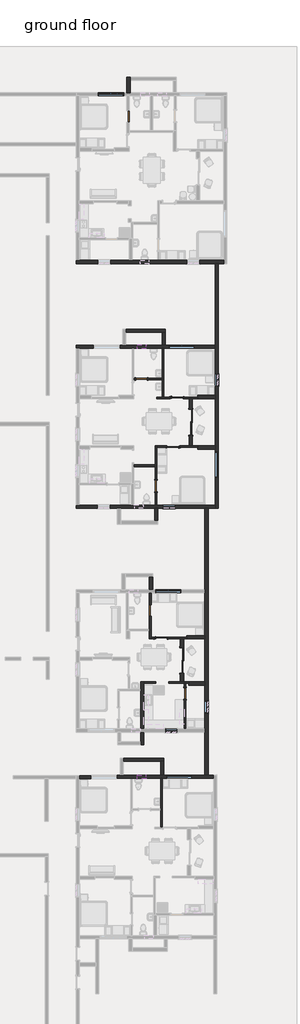
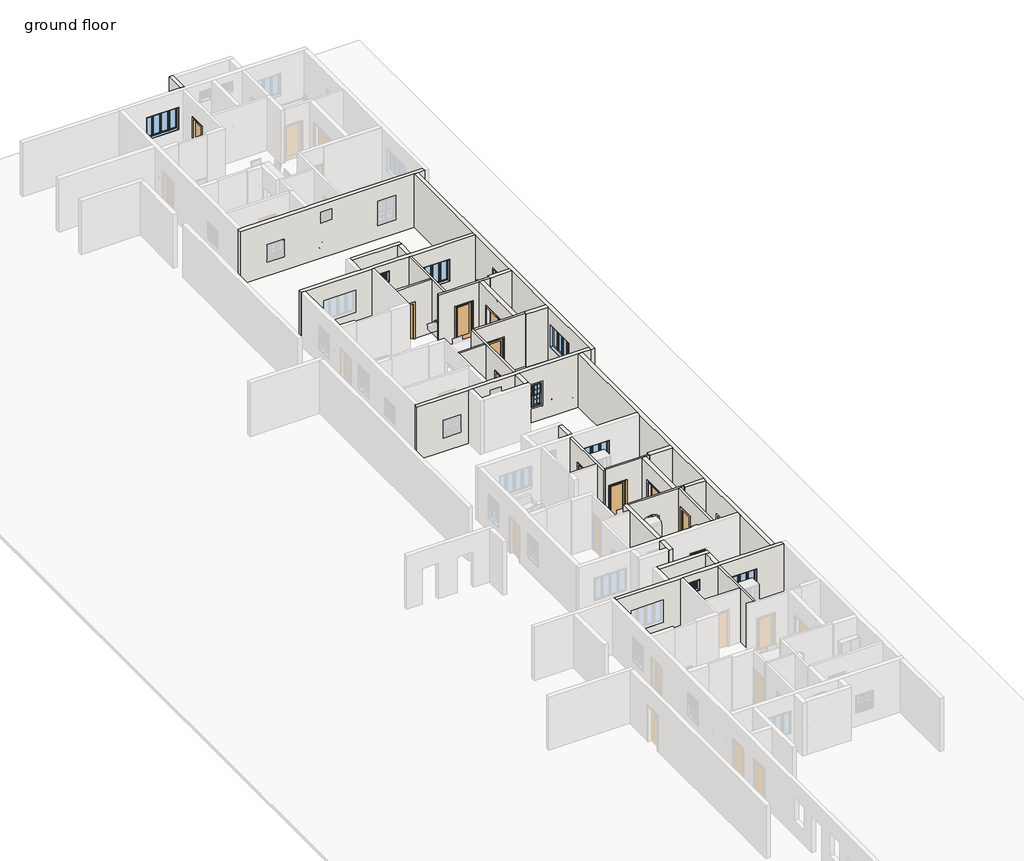
# One storey, part 9 of 16: 32 walls, 11 windows, 10 doors.
# Revit data of these elements (continued)
# Elements 22, 23, 24, 25, 26, 27, 28, 29, 30, 31, 32, 33, 34, 35, 36, 37, 38, 39, 40, 41, 42 (IfcWall, "Generic - 9\"") (continued)
#   Materials on its faces: "Default Wall"
# Element 43 (IfcWindow, "Window-Casement-Double-Awning : 34\" x 36\"")
#   Mark = "74"
#   Window Inset = 0' - 0"
#   Interior Wall Closure = 0' - 2 1/4"
#   Frame Extension = 0' - 0 1/4"
#   Exterior Wall Closure = 0' - 1 1/4"
#   Interior Trim Visibility = yes
#   Exterior Trim Visibility = yes
#   Phase Created = New Construction
#   Materials on its faces: "Wood - Stained", "Glass", "Clad - White"
# Element 44 (IfcWindow, "Window-Casement-Double-Awning : 34\" x 36\"")
#   Mark = "75"
#   Window Inset = 0' - 0"
#   Interior Wall Closure = 0' - 2 1/4"
#   Frame Extension = 0' - 0 1/4"
#   Exterior Wall Closure = 0' - 1 1/4"
#   Interior Trim Visibility = yes
#   Exterior Trim Visibility = yes
#   Phase Created = New Construction
#   Materials on its faces: "Wood - Stained", "Glass", "Clad - White"
# Element 45 (IfcWindow, "Window-Casement-Multi-Sash-Horizontal : 72\" x 53\"")
#   Mark = "17"
#   Window Inset = 0' - 0 5/8"
#   Frame Gap 3 = 0' - 1 83/128"
#   Frame Gap 2 = 0' - 0 5/8"
#   Phase Created = New Construction
#   Materials on its faces: "Metal - Aluminum", "Glass"
# Element 46 (IfcWindow, "Window-Casement-Multi-Sash-Horizontal : 72\" x 53\"")
#   Mark = "21"
#   Window Inset = 0' - 0 5/8"
#   Frame Gap 3 = 0' - 1 83/128"
#   Frame Gap 2 = 0' - 0 5/8"
#   Phase Created = New Construction
#   Materials on its faces: "Metal - Aluminum", "Glass"
# Element 47 (IfcWindow, "Window-Casement-Multi-Sash-Horizontal : 72\" x 53\"")
#   Mark = "22"
#   Window Inset = 0' - 0 5/8"
#   Frame Gap 3 = 0' - 1 83/128"
#   Frame Gap 2 = 0' - 0 5/8"
#   Phase Created = New Construction
#   Materials on its faces: "Metal - Aluminum", "Glass"
# Element 48 (IfcWindow, "Window-Casement-Multi-Sash-Horizontal : 72\" x 53\"")
#   Mark = "23"
#   Window Inset = 0' - 0 5/8"
#   Frame Gap 3 = 0' - 1 83/128"
#   Frame Gap 2 = 0' - 0 5/8"
#   Phase Created = New Construction
#   Materials on its faces: "Metal - Aluminum", "Glass"
# Element 49 (IfcWindow, "Window-Casement-Multi-Sash-Horizontal : 72\" x 53\"")
#   Mark = "27"
#   Window Inset = 0' - 0 5/8"
#   Frame Gap 3 = 0' - 1 83/128"
#   Frame Gap 2 = 0' - 0 5/8"
#   Phase Created = New Construction
#   Materials on its faces: "Metal - Aluminum", "Glass"
# Element 50 (IfcWindow, "Window-Louvers : 24\" x 24\"")
#   Mark = "94"
#   Blade Width = 1' - 10 1/2"
#   Phase Created = New Construction
#   Materials on its faces: "Birch"
# Element 51 (IfcWindow, "Window-Louvers : 24\" x 24\"")
#   Mark = "98"
#   Blade Width = 1' - 10 1/2"
#   Phase Created = New Construction
#   Materials on its faces: "Birch"
# Element 52 (IfcWindow, "Window-Single-Hung-Double : 36\" x 52\"")
#   Mark = "45"
#   Window Inset = 0' - 0"
#   Interior Wall Closure = 0' - 1 1/2"
#   Frame Extension = 0' - 1 1/4"
#   Exterior Wall Closure = 0' - 0 1/2"
#   Interior Trim Visibility = yes
#   Indicator Visibility = yes
#   Exterior Trim Visibility = yes
#   Phase Created = New Construction
#   Materials on its faces: "Wood - Stained", "Glass", "Clad - White"
# Element 53 (IfcWindow, "Window-Single-Hung-Double : 36\" x 52\"")
#   Mark = "47"
#   Window Inset = 0' - 0"
#   Interior Wall Closure = 0' - 1 1/2"
#   Frame Extension = 0' - 1 1/4"
#   Exterior Wall Closure = 0' - 0 1/2"
#   Interior Trim Visibility = yes
#   Indicator Visibility = yes
#   Exterior Trim Visibility = yes
#   Phase Created = New Construction
#   Materials on its faces: "Wood - Stained", "Glass", "Clad - White"
# Materials
#   "Glass": class "Glass", colour RGB 0 128 192, transparency 0.75, Description = "Soda Lime Glass", Cost = 0
#   "Wood - Birch - Solid Stained Light Low Gloss": class "Wood", colour RGB 210 159 95, transparency 0, Cost = 0
#   "Paint - Sienna": colour RGB 118 70 51, transparency 0, Cost = 0
#   "Cherry": class "Wood", colour RGB 226 177 128, transparency 0, Description = "Prunus Serotina", Cost = 0
#   "Aluminum": class "Metal", colour RGB 247 247 247, transparency 0, Description = "Aluminum 6061", Cost = 0
#   "Door - Panel": class "Wood", colour RGB 210 159 95, transparency 0, Cost = 0
#   "Door - Frame": colour RGB 118 70 51, transparency 0, Cost = 0
#   "Wood - Stained": class "Wood", colour RGB 224 178 126, transparency 0, Cost = 0
#   "Clad - White": class "Wood", colour RGB 242 242 238, transparency 0, Cost = 0
#   "Metal - Aluminum": class "Metal", colour RGB 247 247 247, transparency 0
#   "Birch": class "Wood", colour RGB 224 178 126, transparency 0, Description = "Betula Alleghaniensis", Cost = 0
#   "Default Wall": colour RGB 128 128 128, transparency 0, Cost = 0
